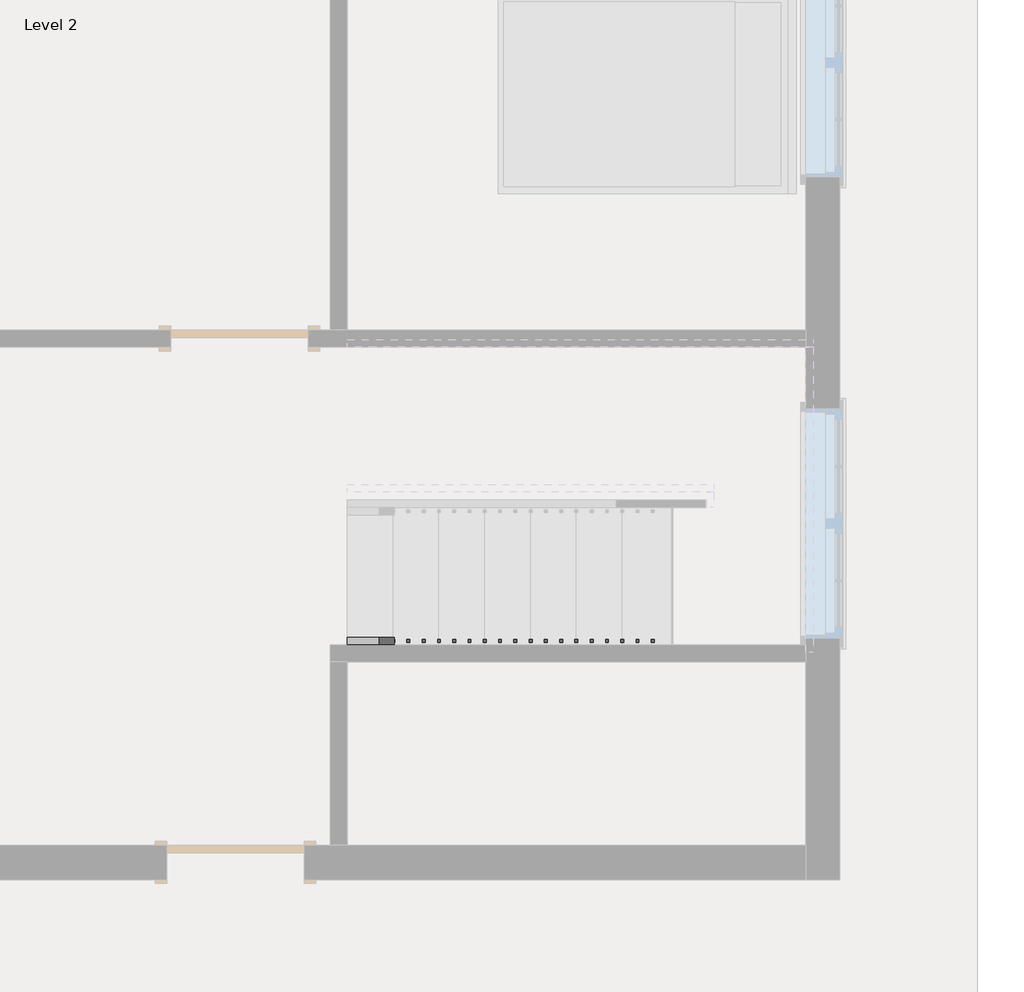
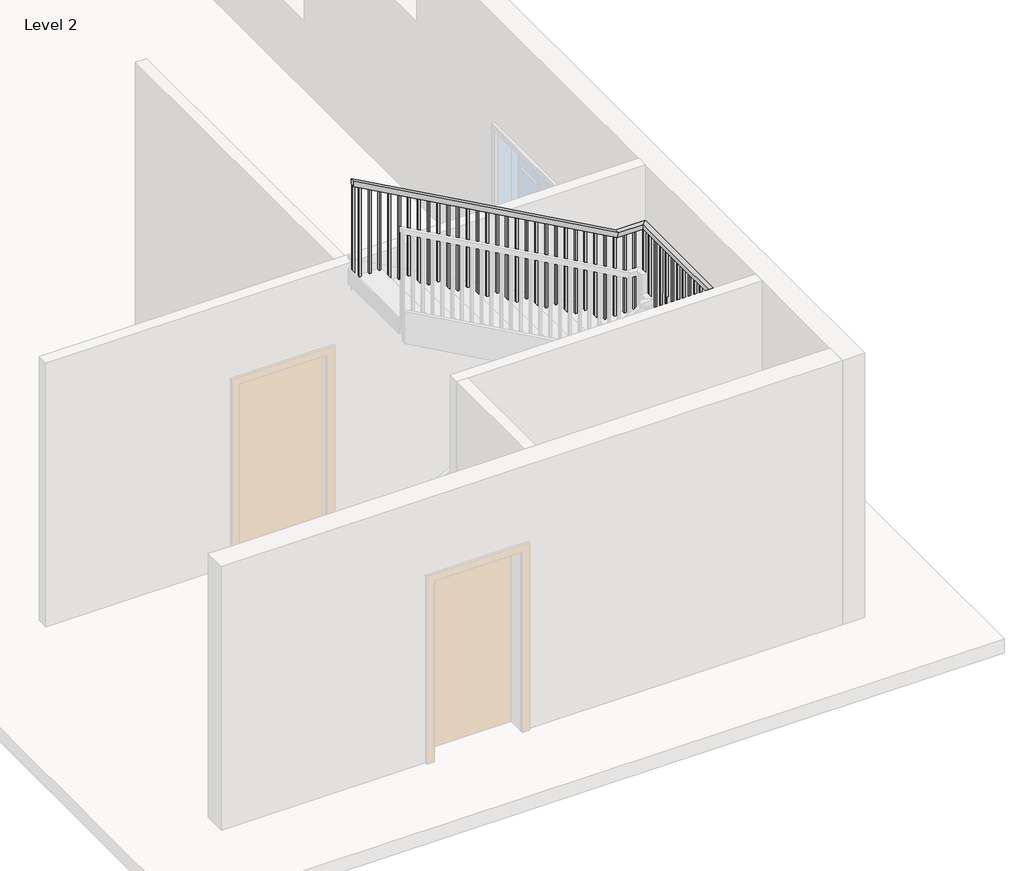
# One storey, part 2 of 3: 1 railing.
"""IFC4 building model written with IfcOpenShell, lengths in millimetres."""

from ifc_helpers import new_model, si_unit, frame, origin, place, context, project, spatial, polyline, outline, extrude, faceted_brep, element, save

model = new_model("IFC4")

# Units and contexts
model_context = context("Model", 3, world=origin())
ifc_project = project(units=[si_unit("LENGTHUNIT", "METRE", prefix="MILLI")], contexts=[model_context])

# Site, building, storey
site = spatial("IfcSite", under=ifc_project)
building = spatial("IfcBuilding", under=site)
storey = spatial("IfcBuildingStorey", under=building, Name="Level 2", Elevation=3048.0)

# Railing
placement = place(None, origin())
element("IfcRailing", 1, ObjectType="Handrail - Rectangular", at=placement, inside=storey, context=model_context, shape_type="SolidModel", body=[
    faceted_brep([(-1197.97188, -4765.70869, 4131.7333333), (-1197.97188, -4765.70869, 4073.620221), (-1197.97188, -4816.50869, 4073.620221), (-1197.97188, -4816.50869, 4131.7333333), (1240.42812, -4765.70869, 5486.4), (1253.5917222, -4765.70869, 5435.6), (1253.5917222, -4816.50869, 5435.6), (1240.42812, -4816.50869, 5486.4), (1799.22812, -4765.70869, 5486.4), (1799.22812, -4765.70869, 5435.6), (1850.02812, -4816.50869, 5435.6), (1850.02812, -4816.50869, 5486.4), (1799.22812, -2886.10869, 5486.4), (1799.22812, -2886.10869, 5435.6), (1850.02812, -2835.30869, 5435.6), (1850.02812, -2835.30869, 5486.4), (1545.22812, -2886.10869, 5486.4), (1532.0645177, -2886.10869, 5435.6), (1532.0645177, -2835.30869, 5435.6), (1545.22812, -2835.30869, 5486.4), (-1197.97188, -2886.10869, 7010.4), (-1197.97188, -2835.30869, 7010.4), (-1197.97188, -2835.30869, 6952.2868876), (-1197.97188, -2886.10869, 6952.2868876)], [[[0, 1, 2, 3]], [[1, 0, 4, 5]], [[2, 1, 5, 6]], [[3, 2, 6, 7]], [[0, 3, 7, 4]], [[5, 4, 8, 9]], [[6, 5, 9, 10]], [[7, 6, 10, 11]], [[4, 7, 11, 8]], [[9, 8, 12, 13]], [[10, 9, 13, 14]], [[11, 10, 14, 15]], [[8, 11, 15, 12]], [[13, 12, 16, 17]], [[14, 13, 17, 18]], [[15, 14, 18, 19]], [[12, 15, 19, 16]], [[20, 21, 22, 23]], [[17, 16, 20, 23]], [[18, 17, 23, 22]], [[19, 18, 22, 21]], [[16, 19, 21, 20]]]),
    extrude(outline(polyline([(6904.6618876, -1112.24688), (6915.245221, -1131.29688), (5926.6666667, -1131.29688), (5926.6666667, -1112.24688), (6904.6618876, -1112.24688)])), frame((0.0, -2870.23369, 0.0), z_axis=(0.0, 1.0, 0.0), x_axis=(0.0, 0.0, 1.0)), (0.0, 0.0, 1.0), 19.05),
    extrude(outline(polyline([(6848.2174432, -1010.64688), (6858.8007765, -1029.69688), (5926.6666667, -1029.69688), (5926.6666667, -1010.64688), (6848.2174432, -1010.64688)])), frame((0.0, -2870.23369, 0.0), z_axis=(0.0, 1.0, 0.0), x_axis=(0.0, 0.0, 1.0)), (0.0, 0.0, 1.0), 19.05),
    extrude(outline(polyline([(6791.7729988, -909.04688), (6802.3563321, -928.09688), (5926.6666667, -928.09688), (5926.6666667, -909.04688), (6791.7729988, -909.04688)])), frame((0.0, -2870.23369, 0.0), z_axis=(0.0, 1.0, 0.0), x_axis=(0.0, 0.0, 1.0)), (0.0, 0.0, 1.0), 19.05),
    extrude(outline(polyline([(6735.3285543, -807.44688), (6745.9118876, -826.49688), (5757.3333333, -826.49688), (5757.3333333, -807.44688), (6735.3285543, -807.44688)])), frame((0.0, -2870.23369, 0.0), z_axis=(0.0, 1.0, 0.0), x_axis=(0.0, 0.0, 1.0)), (0.0, 0.0, 1.0), 19.05),
    extrude(outline(polyline([(6678.8841099, -705.84688), (6689.4674432, -724.89688), (5757.3333333, -724.89688), (5757.3333333, -705.84688), (6678.8841099, -705.84688)])), frame((0.0, -2870.23369, 0.0), z_axis=(0.0, 1.0, 0.0), x_axis=(0.0, 0.0, 1.0)), (0.0, 0.0, 1.0), 19.05),
    extrude(outline(polyline([(6622.4396654, -604.24688), (6633.0229988, -623.29688), (5757.3333333, -623.29688), (5757.3333333, -604.24688), (6622.4396654, -604.24688)])), frame((0.0, -2870.23369, 0.0), z_axis=(0.0, 1.0, 0.0), x_axis=(0.0, 0.0, 1.0)), (0.0, 0.0, 1.0), 19.05),
    extrude(outline(polyline([(6565.995221, -502.64688), (6576.5785543, -521.69688), (5588.0, -521.69688), (5588.0, -502.64688), (6565.995221, -502.64688)])), frame((0.0, -2870.23369, 0.0), z_axis=(0.0, 1.0, 0.0), x_axis=(0.0, 0.0, 1.0)), (0.0, 0.0, 1.0), 19.05),
    extrude(outline(polyline([(6509.5507765, -401.04688), (6520.1341099, -420.09688), (5588.0, -420.09688), (5588.0, -401.04688), (6509.5507765, -401.04688)])), frame((0.0, -2870.23369, 0.0), z_axis=(0.0, 1.0, 0.0), x_axis=(0.0, 0.0, 1.0)), (0.0, 0.0, 1.0), 19.05),
    extrude(outline(polyline([(6453.1063321, -299.44688), (6463.6896654, -318.49688), (5588.0, -318.49688), (5588.0, -299.44688), (6453.1063321, -299.44688)])), frame((0.0, -2870.23369, 0.0), z_axis=(0.0, 1.0, 0.0), x_axis=(0.0, 0.0, 1.0)), (0.0, 0.0, 1.0), 19.05),
    extrude(outline(polyline([(6396.6618876, -197.84688), (6407.245221, -216.89688), (5418.6666667, -216.89688), (5418.6666667, -197.84688), (6396.6618876, -197.84688)])), frame((0.0, -2870.23369, 0.0), z_axis=(0.0, 1.0, 0.0), x_axis=(0.0, 0.0, 1.0)), (0.0, 0.0, 1.0), 19.05),
    extrude(outline(polyline([(6340.2174432, -96.24688), (6350.8007765, -115.29688), (5418.6666667, -115.29688), (5418.6666667, -96.24688), (6340.2174432, -96.24688)])), frame((0.0, -2870.23369, 0.0), z_axis=(0.0, 1.0, 0.0), x_axis=(0.0, 0.0, 1.0)), (0.0, 0.0, 1.0), 19.05),
    extrude(outline(polyline([(6283.7729988, 5.35312), (6294.3563321, -13.69688), (5418.6666667, -13.69688), (5418.6666667, 5.35312), (6283.7729988, 5.35312)])), frame((0.0, -2870.23369, 0.0), z_axis=(0.0, 1.0, 0.0), x_axis=(0.0, 0.0, 1.0)), (0.0, 0.0, 1.0), 19.05),
    extrude(outline(polyline([(6227.3285543, 106.95312), (6237.9118876, 87.90312), (5249.3333333, 87.90312), (5249.3333333, 106.95312), (6227.3285543, 106.95312)])), frame((0.0, -2870.23369, 0.0), z_axis=(0.0, 1.0, 0.0), x_axis=(0.0, 0.0, 1.0)), (0.0, 0.0, 1.0), 19.05),
    extrude(outline(polyline([(6170.8841099, 208.55312), (6181.4674432, 189.50312), (5249.3333333, 189.50312), (5249.3333333, 208.55312), (6170.8841099, 208.55312)])), frame((0.0, -2870.23369, 0.0), z_axis=(0.0, 1.0, 0.0), x_axis=(0.0, 0.0, 1.0)), (0.0, 0.0, 1.0), 19.05),
    extrude(outline(polyline([(6114.4396654, 310.15312), (6125.0229988, 291.10312), (5249.3333333, 291.10312), (5249.3333333, 310.15312), (6114.4396654, 310.15312)])), frame((0.0, -2870.23369, 0.0), z_axis=(0.0, 1.0, 0.0), x_axis=(0.0, 0.0, 1.0)), (0.0, 0.0, 1.0), 19.05),
    extrude(outline(polyline([(6057.995221, 411.75312), (6068.5785543, 392.70312), (5080.0, 392.70312), (5080.0, 411.75312), (6057.995221, 411.75312)])), frame((0.0, -2870.23369, 0.0), z_axis=(0.0, 1.0, 0.0), x_axis=(0.0, 0.0, 1.0)), (0.0, 0.0, 1.0), 19.05),
    extrude(outline(polyline([(6001.5507765, 513.35312), (6012.1341099, 494.30312), (5080.0, 494.30312), (5080.0, 513.35312), (6001.5507765, 513.35312)])), frame((0.0, -2870.23369, 0.0), z_axis=(0.0, 1.0, 0.0), x_axis=(0.0, 0.0, 1.0)), (0.0, 0.0, 1.0), 19.05),
    extrude(outline(polyline([(5945.1063321, 614.95312), (5955.6896654, 595.90312), (5080.0, 595.90312), (5080.0, 614.95312), (5945.1063321, 614.95312)])), frame((0.0, -2870.23369, 0.0), z_axis=(0.0, 1.0, 0.0), x_axis=(0.0, 0.0, 1.0)), (0.0, 0.0, 1.0), 19.05),
    extrude(outline(polyline([(5888.6618876, 716.55312), (5899.245221, 697.50312), (4910.6666667, 697.50312), (4910.6666667, 716.55312), (5888.6618876, 716.55312)])), frame((0.0, -2870.23369, 0.0), z_axis=(0.0, 1.0, 0.0), x_axis=(0.0, 0.0, 1.0)), (0.0, 0.0, 1.0), 19.05),
    extrude(outline(polyline([(5832.2174432, 818.15312), (5842.8007765, 799.10312), (4910.6666667, 799.10312), (4910.6666667, 818.15312), (5832.2174432, 818.15312)])), frame((0.0, -2870.23369, 0.0), z_axis=(0.0, 1.0, 0.0), x_axis=(0.0, 0.0, 1.0)), (0.0, 0.0, 1.0), 19.05),
    extrude(outline(polyline([(5775.7729988, 919.75312), (5786.3563321, 900.70312), (4910.6666667, 900.70312), (4910.6666667, 919.75312), (5775.7729988, 919.75312)])), frame((0.0, -2870.23369, 0.0), z_axis=(0.0, 1.0, 0.0), x_axis=(0.0, 0.0, 1.0)), (0.0, 0.0, 1.0), 19.05),
    extrude(outline(polyline([(5719.3285543, 1021.35312), (5729.9118876, 1002.30312), (4741.3333333, 1002.30312), (4741.3333333, 1021.35312), (5719.3285543, 1021.35312)])), frame((0.0, -2870.23369, 0.0), z_axis=(0.0, 1.0, 0.0), x_axis=(0.0, 0.0, 1.0)), (0.0, 0.0, 1.0), 19.05),
    extrude(outline(polyline([(5662.8841099, 1122.95312), (5673.4674432, 1103.90312), (4741.3333333, 1103.90312), (4741.3333333, 1122.95312), (5662.8841099, 1122.95312)])), frame((0.0, -2870.23369, 0.0), z_axis=(0.0, 1.0, 0.0), x_axis=(0.0, 0.0, 1.0)), (0.0, 0.0, 1.0), 19.05),
    extrude(outline(polyline([(5606.4396654, 1224.55312), (5617.0229988, 1205.50312), (4741.3333333, 1205.50312), (4741.3333333, 1224.55312), (5606.4396654, 1224.55312)])), frame((0.0, -2870.23369, 0.0), z_axis=(0.0, 1.0, 0.0), x_axis=(0.0, 0.0, 1.0)), (0.0, 0.0, 1.0), 19.05),
    extrude(outline(polyline([(5549.995221, 1326.15312), (5560.5785543, 1307.10312), (4572.0, 1307.10312), (4572.0, 1326.15312), (5549.995221, 1326.15312)])), frame((0.0, -2870.23369, 0.0), z_axis=(0.0, 1.0, 0.0), x_axis=(0.0, 0.0, 1.0)), (0.0, 0.0, 1.0), 19.05),
    extrude(outline(polyline([(5493.5507765, 1427.75312), (5504.1341099, 1408.70312), (4572.0, 1408.70312), (4572.0, 1427.75312), (5493.5507765, 1427.75312)])), frame((0.0, -2870.23369, 0.0), z_axis=(0.0, 1.0, 0.0), x_axis=(0.0, 0.0, 1.0)), (0.0, 0.0, 1.0), 19.05),
    extrude(outline(polyline([(5437.1063321, 1529.35312), (5447.6896654, 1510.30312), (4572.0, 1510.30312), (4572.0, 1529.35312), (5437.1063321, 1529.35312)])), frame((0.0, -2870.23369, 0.0), z_axis=(0.0, 1.0, 0.0), x_axis=(0.0, 0.0, 1.0)), (0.0, 0.0, 1.0), 19.05),
    extrude(outline(polyline([(1630.95312, -2851.18369), (1630.95312, -2870.23369), (1611.90312, -2870.23369), (1611.90312, -2851.18369), (1630.95312, -2851.18369)])), frame((0.0, 0.0, 4572.0), z_axis=(0.0, 0.0, 1.0), x_axis=(1.0, 0.0, 0.0)), (0.0, 0.0, 1.0), 863.6),
    extrude(outline(polyline([(1732.55312, -2851.18369), (1732.55312, -2870.23369), (1713.50312, -2870.23369), (1713.50312, -2851.18369), (1732.55312, -2851.18369)])), frame((0.0, 0.0, 4572.0), z_axis=(0.0, 0.0, 1.0), x_axis=(1.0, 0.0, 0.0)), (0.0, 0.0, 1.0), 863.6),
    extrude(outline(polyline([(1834.15312, -2971.83369), (1815.10312, -2971.83369), (1815.10312, -2952.78369), (1834.15312, -2952.78369), (1834.15312, -2971.83369)])), frame((0.0, 0.0, 4572.0), z_axis=(0.0, 0.0, 1.0), x_axis=(1.0, 0.0, 0.0)), (0.0, 0.0, 1.0), 863.6),
    extrude(outline(polyline([(1834.15312, -3073.43369), (1815.10312, -3073.43369), (1815.10312, -3054.38369), (1834.15312, -3054.38369), (1834.15312, -3073.43369)])), frame((0.0, 0.0, 4572.0), z_axis=(0.0, 0.0, 1.0), x_axis=(1.0, 0.0, 0.0)), (0.0, 0.0, 1.0), 863.6),
    extrude(outline(polyline([(1834.15312, -3175.03369), (1815.10312, -3175.03369), (1815.10312, -3155.98369), (1834.15312, -3155.98369), (1834.15312, -3175.03369)])), frame((0.0, 0.0, 4572.0), z_axis=(0.0, 0.0, 1.0), x_axis=(1.0, 0.0, 0.0)), (0.0, 0.0, 1.0), 863.6),
    extrude(outline(polyline([(1834.15312, -3276.63369), (1815.10312, -3276.63369), (1815.10312, -3257.58369), (1834.15312, -3257.58369), (1834.15312, -3276.63369)])), frame((0.0, 0.0, 4572.0), z_axis=(0.0, 0.0, 1.0), x_axis=(1.0, 0.0, 0.0)), (0.0, 0.0, 1.0), 863.6),
    extrude(outline(polyline([(1834.15312, -3378.23369), (1815.10312, -3378.23369), (1815.10312, -3359.18369), (1834.15312, -3359.18369), (1834.15312, -3378.23369)])), frame((0.0, 0.0, 4572.0), z_axis=(0.0, 0.0, 1.0), x_axis=(1.0, 0.0, 0.0)), (0.0, 0.0, 1.0), 863.6),
    extrude(outline(polyline([(1834.15312, -3479.83369), (1815.10312, -3479.83369), (1815.10312, -3460.78369), (1834.15312, -3460.78369), (1834.15312, -3479.83369)])), frame((0.0, 0.0, 4572.0), z_axis=(0.0, 0.0, 1.0), x_axis=(1.0, 0.0, 0.0)), (0.0, 0.0, 1.0), 863.6),
    extrude(outline(polyline([(1834.15312, -3581.43369), (1815.10312, -3581.43369), (1815.10312, -3562.38369), (1834.15312, -3562.38369), (1834.15312, -3581.43369)])), frame((0.0, 0.0, 4572.0), z_axis=(0.0, 0.0, 1.0), x_axis=(1.0, 0.0, 0.0)), (0.0, 0.0, 1.0), 863.6),
    extrude(outline(polyline([(1834.15312, -3683.03369), (1815.10312, -3683.03369), (1815.10312, -3663.98369), (1834.15312, -3663.98369), (1834.15312, -3683.03369)])), frame((0.0, 0.0, 4572.0), z_axis=(0.0, 0.0, 1.0), x_axis=(1.0, 0.0, 0.0)), (0.0, 0.0, 1.0), 863.6),
    extrude(outline(polyline([(1834.15312, -3784.63369), (1815.10312, -3784.63369), (1815.10312, -3765.58369), (1834.15312, -3765.58369), (1834.15312, -3784.63369)])), frame((0.0, 0.0, 4572.0), z_axis=(0.0, 0.0, 1.0), x_axis=(1.0, 0.0, 0.0)), (0.0, 0.0, 1.0), 863.6),
    extrude(outline(polyline([(1834.15312, -3886.23369), (1815.10312, -3886.23369), (1815.10312, -3867.18369), (1834.15312, -3867.18369), (1834.15312, -3886.23369)])), frame((0.0, 0.0, 4572.0), z_axis=(0.0, 0.0, 1.0), x_axis=(1.0, 0.0, 0.0)), (0.0, 0.0, 1.0), 863.6),
    extrude(outline(polyline([(1834.15312, -3987.83369), (1815.10312, -3987.83369), (1815.10312, -3968.78369), (1834.15312, -3968.78369), (1834.15312, -3987.83369)])), frame((0.0, 0.0, 4572.0), z_axis=(0.0, 0.0, 1.0), x_axis=(1.0, 0.0, 0.0)), (0.0, 0.0, 1.0), 863.6),
    extrude(outline(polyline([(1834.15312, -4089.43369), (1815.10312, -4089.43369), (1815.10312, -4070.38369), (1834.15312, -4070.38369), (1834.15312, -4089.43369)])), frame((0.0, 0.0, 4572.0), z_axis=(0.0, 0.0, 1.0), x_axis=(1.0, 0.0, 0.0)), (0.0, 0.0, 1.0), 863.6),
    extrude(outline(polyline([(1834.15312, -4191.03369), (1815.10312, -4191.03369), (1815.10312, -4171.98369), (1834.15312, -4171.98369), (1834.15312, -4191.03369)])), frame((0.0, 0.0, 4572.0), z_axis=(0.0, 0.0, 1.0), x_axis=(1.0, 0.0, 0.0)), (0.0, 0.0, 1.0), 863.6),
    extrude(outline(polyline([(1834.15312, -4292.63369), (1815.10312, -4292.63369), (1815.10312, -4273.58369), (1834.15312, -4273.58369), (1834.15312, -4292.63369)])), frame((0.0, 0.0, 4572.0), z_axis=(0.0, 0.0, 1.0), x_axis=(1.0, 0.0, 0.0)), (0.0, 0.0, 1.0), 863.6),
    extrude(outline(polyline([(1834.15312, -4394.23369), (1815.10312, -4394.23369), (1815.10312, -4375.18369), (1834.15312, -4375.18369), (1834.15312, -4394.23369)])), frame((0.0, 0.0, 4572.0), z_axis=(0.0, 0.0, 1.0), x_axis=(1.0, 0.0, 0.0)), (0.0, 0.0, 1.0), 863.6),
    extrude(outline(polyline([(1834.15312, -4495.83369), (1815.10312, -4495.83369), (1815.10312, -4476.78369), (1834.15312, -4476.78369), (1834.15312, -4495.83369)])), frame((0.0, 0.0, 4572.0), z_axis=(0.0, 0.0, 1.0), x_axis=(1.0, 0.0, 0.0)), (0.0, 0.0, 1.0), 863.6),
    extrude(outline(polyline([(1834.15312, -4597.43369), (1815.10312, -4597.43369), (1815.10312, -4578.38369), (1834.15312, -4578.38369), (1834.15312, -4597.43369)])), frame((0.0, 0.0, 4572.0), z_axis=(0.0, 0.0, 1.0), x_axis=(1.0, 0.0, 0.0)), (0.0, 0.0, 1.0), 863.6),
    extrude(outline(polyline([(1834.15312, -4699.03369), (1815.10312, -4699.03369), (1815.10312, -4679.98369), (1834.15312, -4679.98369), (1834.15312, -4699.03369)])), frame((0.0, 0.0, 4572.0), z_axis=(0.0, 0.0, 1.0), x_axis=(1.0, 0.0, 0.0)), (0.0, 0.0, 1.0), 863.6),
    extrude(outline(polyline([(1738.90312, -4800.63369), (1738.90312, -4781.58369), (1757.95312, -4781.58369), (1757.95312, -4800.63369), (1738.90312, -4800.63369)])), frame((0.0, 0.0, 4572.0), z_axis=(0.0, 0.0, 1.0), x_axis=(1.0, 0.0, 0.0)), (0.0, 0.0, 1.0), 863.6),
    extrude(outline(polyline([(1637.30312, -4800.63369), (1637.30312, -4781.58369), (1656.35312, -4781.58369), (1656.35312, -4800.63369), (1637.30312, -4800.63369)])), frame((0.0, 0.0, 4572.0), z_axis=(0.0, 0.0, 1.0), x_axis=(1.0, 0.0, 0.0)), (0.0, 0.0, 1.0), 863.6),
    extrude(outline(polyline([(1535.70312, -4800.63369), (1535.70312, -4781.58369), (1554.75312, -4781.58369), (1554.75312, -4800.63369), (1535.70312, -4800.63369)])), frame((0.0, 0.0, 4572.0), z_axis=(0.0, 0.0, 1.0), x_axis=(1.0, 0.0, 0.0)), (0.0, 0.0, 1.0), 863.6),
    extrude(outline(polyline([(1434.10312, -4800.63369), (1434.10312, -4781.58369), (1453.15312, -4781.58369), (1453.15312, -4800.63369), (1434.10312, -4800.63369)])), frame((0.0, 0.0, 4572.0), z_axis=(0.0, 0.0, 1.0), x_axis=(1.0, 0.0, 0.0)), (0.0, 0.0, 1.0), 863.6),
    extrude(outline(polyline([(1332.50312, -4800.63369), (1332.50312, -4781.58369), (1351.55312, -4781.58369), (1351.55312, -4800.63369), (1332.50312, -4800.63369)])), frame((0.0, 0.0, 4572.0), z_axis=(0.0, 0.0, 1.0), x_axis=(1.0, 0.0, 0.0)), (0.0, 0.0, 1.0), 863.6),
    extrude(outline(polyline([(5433.5785543, 1249.95312), (5422.995221, 1230.90312), (4572.0, 1230.90312), (4572.0, 1249.95312), (5433.5785543, 1249.95312)])), frame((0.0, -4800.63369, 0.0), z_axis=(0.0, 1.0, 0.0), x_axis=(0.0, 0.0, 1.0)), (0.0, 0.0, 1.0), 19.05),
    extrude(outline(polyline([(5377.1341099, 1148.35312), (5366.5507765, 1129.30312), (4402.6666667, 1129.30312), (4402.6666667, 1148.35312), (5377.1341099, 1148.35312)])), frame((0.0, -4800.63369, 0.0), z_axis=(0.0, 1.0, 0.0), x_axis=(0.0, 0.0, 1.0)), (0.0, 0.0, 1.0), 19.05),
    extrude(outline(polyline([(5320.6896654, 1046.75312), (5310.1063321, 1027.70312), (4402.6666667, 1027.70312), (4402.6666667, 1046.75312), (5320.6896654, 1046.75312)])), frame((0.0, -4800.63369, 0.0), z_axis=(0.0, 1.0, 0.0), x_axis=(0.0, 0.0, 1.0)), (0.0, 0.0, 1.0), 19.05),
    extrude(outline(polyline([(5264.245221, 945.15312), (5253.6618876, 926.10312), (4402.6666667, 926.10312), (4402.6666667, 945.15312), (5264.245221, 945.15312)])), frame((0.0, -4800.63369, 0.0), z_axis=(0.0, 1.0, 0.0), x_axis=(0.0, 0.0, 1.0)), (0.0, 0.0, 1.0), 19.05),
    extrude(outline(polyline([(5207.8007765, 843.55312), (5197.2174432, 824.50312), (4233.3333333, 824.50312), (4233.3333333, 843.55312), (5207.8007765, 843.55312)])), frame((0.0, -4800.63369, 0.0), z_axis=(0.0, 1.0, 0.0), x_axis=(0.0, 0.0, 1.0)), (0.0, 0.0, 1.0), 19.05),
    extrude(outline(polyline([(5151.3563321, 741.95312), (5140.7729988, 722.90312), (4233.3333333, 722.90312), (4233.3333333, 741.95312), (5151.3563321, 741.95312)])), frame((0.0, -4800.63369, 0.0), z_axis=(0.0, 1.0, 0.0), x_axis=(0.0, 0.0, 1.0)), (0.0, 0.0, 1.0), 19.05),
    extrude(outline(polyline([(5094.9118876, 640.35312), (5084.3285543, 621.30312), (4233.3333333, 621.30312), (4233.3333333, 640.35312), (5094.9118876, 640.35312)])), frame((0.0, -4800.63369, 0.0), z_axis=(0.0, 1.0, 0.0), x_axis=(0.0, 0.0, 1.0)), (0.0, 0.0, 1.0), 19.05),
    extrude(outline(polyline([(5038.4674432, 538.75312), (5027.8841099, 519.70312), (4064.0, 519.70312), (4064.0, 538.75312), (5038.4674432, 538.75312)])), frame((0.0, -4800.63369, 0.0), z_axis=(0.0, 1.0, 0.0), x_axis=(0.0, 0.0, 1.0)), (0.0, 0.0, 1.0), 19.05),
    extrude(outline(polyline([(4982.0229988, 437.15312), (4971.4396654, 418.10312), (4064.0, 418.10312), (4064.0, 437.15312), (4982.0229988, 437.15312)])), frame((0.0, -4800.63369, 0.0), z_axis=(0.0, 1.0, 0.0), x_axis=(0.0, 0.0, 1.0)), (0.0, 0.0, 1.0), 19.05),
    extrude(outline(polyline([(4925.5785543, 335.55312), (4914.995221, 316.50312), (4064.0, 316.50312), (4064.0, 335.55312), (4925.5785543, 335.55312)])), frame((0.0, -4800.63369, 0.0), z_axis=(0.0, 1.0, 0.0), x_axis=(0.0, 0.0, 1.0)), (0.0, 0.0, 1.0), 19.05),
    extrude(outline(polyline([(4869.1341099, 233.95312), (4858.5507765, 214.90312), (3894.6666667, 214.90312), (3894.6666667, 233.95312), (4869.1341099, 233.95312)])), frame((0.0, -4800.63369, 0.0), z_axis=(0.0, 1.0, 0.0), x_axis=(0.0, 0.0, 1.0)), (0.0, 0.0, 1.0), 19.05),
    extrude(outline(polyline([(4812.6896654, 132.35312), (4802.1063321, 113.30312), (3894.6666667, 113.30312), (3894.6666667, 132.35312), (4812.6896654, 132.35312)])), frame((0.0, -4800.63369, 0.0), z_axis=(0.0, 1.0, 0.0), x_axis=(0.0, 0.0, 1.0)), (0.0, 0.0, 1.0), 19.05),
    extrude(outline(polyline([(4756.245221, 30.75312), (4745.6618876, 11.70312), (3894.6666667, 11.70312), (3894.6666667, 30.75312), (4756.245221, 30.75312)])), frame((0.0, -4800.63369, 0.0), z_axis=(0.0, 1.0, 0.0), x_axis=(0.0, 0.0, 1.0)), (0.0, 0.0, 1.0), 19.05),
    extrude(outline(polyline([(4699.8007765, -70.84688), (4689.2174432, -89.89688), (3725.3333333, -89.89688), (3725.3333333, -70.84688), (4699.8007765, -70.84688)])), frame((0.0, -4800.63369, 0.0), z_axis=(0.0, 1.0, 0.0), x_axis=(0.0, 0.0, 1.0)), (0.0, 0.0, 1.0), 19.05),
    extrude(outline(polyline([(4643.3563321, -172.44688), (4632.7729988, -191.49688), (3725.3333333, -191.49688), (3725.3333333, -172.44688), (4643.3563321, -172.44688)])), frame((0.0, -4800.63369, 0.0), z_axis=(0.0, 1.0, 0.0), x_axis=(0.0, 0.0, 1.0)), (0.0, 0.0, 1.0), 19.05),
    extrude(outline(polyline([(4586.9118876, -274.04688), (4576.3285543, -293.09688), (3725.3333333, -293.09688), (3725.3333333, -274.04688), (4586.9118876, -274.04688)])), frame((0.0, -4800.63369, 0.0), z_axis=(0.0, 1.0, 0.0), x_axis=(0.0, 0.0, 1.0)), (0.0, 0.0, 1.0), 19.05),
    extrude(outline(polyline([(4530.4674432, -375.64688), (4519.8841099, -394.69688), (3556.0, -394.69688), (3556.0, -375.64688), (4530.4674432, -375.64688)])), frame((0.0, -4800.63369, 0.0), z_axis=(0.0, 1.0, 0.0), x_axis=(0.0, 0.0, 1.0)), (0.0, 0.0, 1.0), 19.05),
    extrude(outline(polyline([(4474.0229988, -477.24688), (4463.4396654, -496.29688), (3556.0, -496.29688), (3556.0, -477.24688), (4474.0229988, -477.24688)])), frame((0.0, -4800.63369, 0.0), z_axis=(0.0, 1.0, 0.0), x_axis=(0.0, 0.0, 1.0)), (0.0, 0.0, 1.0), 19.05),
    extrude(outline(polyline([(4417.5785543, -578.84688), (4406.995221, -597.89688), (3556.0, -597.89688), (3556.0, -578.84688), (4417.5785543, -578.84688)])), frame((0.0, -4800.63369, 0.0), z_axis=(0.0, 1.0, 0.0), x_axis=(0.0, 0.0, 1.0)), (0.0, 0.0, 1.0), 19.05),
    extrude(outline(polyline([(4361.1341099, -680.44688), (4350.5507765, -699.49688), (3386.6666667, -699.49688), (3386.6666667, -680.44688), (4361.1341099, -680.44688)])), frame((0.0, -4800.63369, 0.0), z_axis=(0.0, 1.0, 0.0), x_axis=(0.0, 0.0, 1.0)), (0.0, 0.0, 1.0), 19.05),
    extrude(outline(polyline([(4304.6896654, -782.04688), (4294.1063321, -801.09688), (3386.6666667, -801.09688), (3386.6666667, -782.04688), (4304.6896654, -782.04688)])), frame((0.0, -4800.63369, 0.0), z_axis=(0.0, 1.0, 0.0), x_axis=(0.0, 0.0, 1.0)), (0.0, 0.0, 1.0), 19.05),
    extrude(outline(polyline([(4248.245221, -883.64688), (4237.6618876, -902.69688), (3386.6666667, -902.69688), (3386.6666667, -883.64688), (4248.245221, -883.64688)])), frame((0.0, -4800.63369, 0.0), z_axis=(0.0, 1.0, 0.0), x_axis=(0.0, 0.0, 1.0)), (0.0, 0.0, 1.0), 19.05),
    extrude(outline(polyline([(4191.8007765, -985.24688), (4181.2174432, -1004.29688), (3217.3333333, -1004.29688), (3217.3333333, -985.24688), (4191.8007765, -985.24688)])), frame((0.0, -4800.63369, 0.0), z_axis=(0.0, 1.0, 0.0), x_axis=(0.0, 0.0, 1.0)), (0.0, 0.0, 1.0), 19.05),
    extrude(outline(polyline([(4135.3563321, -1086.84688), (4124.7729988, -1105.89688), (3217.3333333, -1105.89688), (3217.3333333, -1086.84688), (4135.3563321, -1086.84688)])), frame((0.0, -4800.63369, 0.0), z_axis=(0.0, 1.0, 0.0), x_axis=(0.0, 0.0, 1.0)), (0.0, 0.0, 1.0), 19.05),
    extrude(outline(polyline([(1834.15312, -2870.23369), (1815.10312, -2870.23369), (1815.10312, -2851.18369), (1834.15312, -2851.18369), (1834.15312, -2870.23369)])), frame((0.0, 0.0, 4572.0), z_axis=(0.0, 0.0, 1.0), x_axis=(1.0, 0.0, 0.0)), (0.0, 0.0, 1.0), 863.6),
    extrude(outline(polyline([(1815.10312, -4800.63369), (1815.10312, -4781.58369), (1834.15312, -4781.58369), (1834.15312, -4800.63369), (1815.10312, -4800.63369)])), frame((0.0, 0.0, 4572.0), z_axis=(0.0, 0.0, 1.0), x_axis=(1.0, 0.0, 0.0)), (0.0, 0.0, 1.0), 863.6),
    extrude(outline(polyline([(6941.7035543, -1178.92188), (6952.2868876, -1197.97188), (5926.6666667, -1197.97188), (5926.6666667, -1178.92188), (6941.7035543, -1178.92188)])), frame((0.0, -2870.23369, 0.0), z_axis=(0.0, 1.0, 0.0), x_axis=(0.0, 0.0, 1.0)), (0.0, 0.0, 1.0), 19.05),
    extrude(outline(polyline([(4084.2035543, -1178.92188), (4073.620221, -1197.97188), (3217.3333333, -1197.97188), (3217.3333333, -1178.92188), (4084.2035543, -1178.92188)])), frame((0.0, -4800.63369, 0.0), z_axis=(0.0, 1.0, 0.0), x_axis=(0.0, 0.0, 1.0)), (0.0, 0.0, 1.0), 19.05),
])

save(model, "model.ifc")

# Revit data of these elements
# Type "Handrail - Rectangular"
#   Assembly Code = "C2010400"
#   built-in parameter 1008612 = 0.0416667 (stored number, unit not read)
#   built-in parameter 1008611 = 0.0416667 (stored number, unit not read)
#   built-in parameter 1008609 = 0.333333 (stored number, unit not read)
#   built-in parameter 1008604 = 0.166667 (stored number, unit not read)
#   built-in parameter 1008603 = 0.166667 (stored number, unit not read)
#   Railing Height = 3' - 0"
#   built-in parameter 1008630 = 2
#   built-in parameter 1008610 = 2
#   built-in parameter 1008618 = Baluster - Square : 3/4"
# Element 1 (IfcRailing, "Handrail - Rectangular")
#   Phase Created = New Construction
